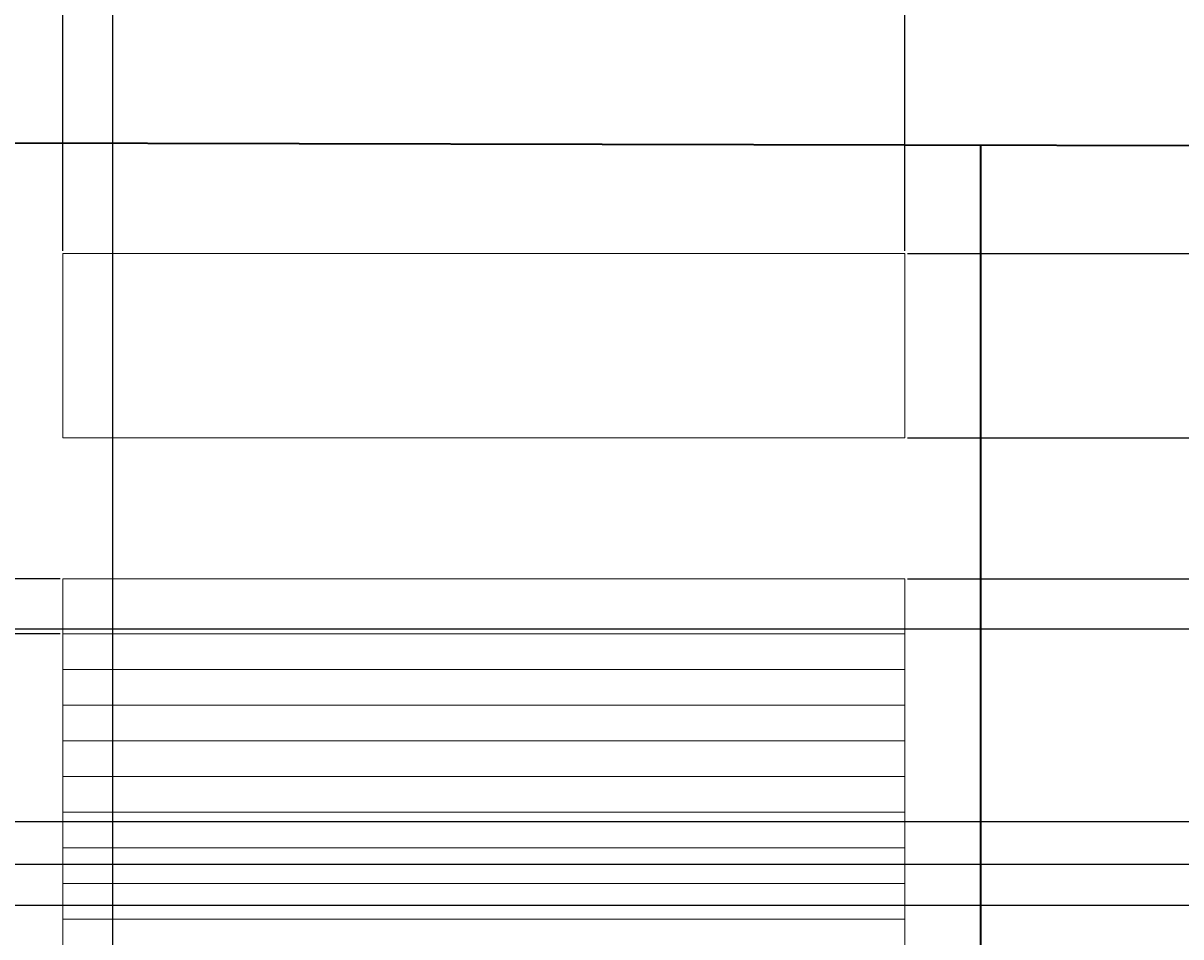
# Model space of a CAD drawing. Units: inches. Extents: x 27 to 200, y -50 to 102.
# Tile 13 of 26: x 144 to 172, y -3 to 19. Entities that reach past the tile are written whole.
import ezdxf

# ---------------------------------------------------------------- set-up
doc = ezdxf.new("R2010")
doc.units = ezdxf.units.IN
doc.header["$MEASUREMENT"] = 0
for name, color, linetype, lineweight in [('A-ANNO-DIMS', 2, 'Continuous', 18), ('A-ELEV', 7, 'Continuous', 35), ('A-EQPM', 9, 'Continuous', 18), ('A-FURN', 8, 'Continuous', 18)]:
    doc.layers.add(name, color=color, linetype=linetype, lineweight=lineweight)
doc.styles.get("Standard").update_dxf_attribs({"font": 'arial.ttf'})
doc.dimstyles.get("Standard").update_dxf_attribs({"dimtxt": 0.18, "dimasz": 0.18, "dimexe": 0.18, "dimexo": 0.0625, "dimgap": 0.09, "dimtad": 0, "dimtih": 1, "dimtoh": 1, "dimdec": 4, "dimzin": 0, "dimdsep": 46, "dimtxsty": 'Standard', "dimcen": 0.09, "dimadec": 0, "dimazin": 0, "dimtfac": 1, "dimtdec": 4, "dimtofl": 0, "dimtmove": 0, "dimatfit": 3, "dimfxl": 1, "dimtolj": 1, "dimtzin": 0, "dimarcsym": 0})

# ---------------------------------------------------------------- blocks, each defined once
blk = doc.blocks.new('*D48')
at = {"layer": 'A-ANNO-DIMS', "color": 0, "lineweight": -2, "transparency": 16777216}
for p, q in [((84.479, 44.926), (199.797, 44.926)), ((199.617, 44.746), (199.617, 14.26)), ((199.617, -16.589), (199.617, 13.897)), ((84.479, -16.769), (199.797, -16.769))]:
    blk.add_line(p, q, dxfattribs=at)
at = {"layer": 'A-ANNO-DIMS', "color": 0, "transparency": 16777216}
for points in [[(199.587, 44.746), (199.647, 44.746), (199.617, 44.926)], [(199.587, -16.589), (199.647, -16.589), (199.617, -16.769)]]:
    blk.add_solid(points, dxfattribs=at)
at = {"layer": 'Defpoints', "color": 0, "transparency": 16777216}
for p in [(84.417, 44.926), (199.617, 44.926), (84.417, -16.769)]:
    blk.add_point(p, dxfattribs=at)
at = {"layer": 'A-ANNO-DIMS', "color": 0, "transparency": 16777216, "insert": (199.617, 14.079), "char_height": 0.18, "attachment_point": 5}
blk.add_mtext('\\A1;61.7', dxfattribs=at)
blk = doc.blocks.new('*D51')
at = {"layer": 'A-ANNO-DIMS', "color": 0, "lineweight": -2, "transparency": 16777216}
for p, q in [((120.417, 45.561), (120.417, -25.149)), ((146.417, 45.561), (146.417, -25.149)), ((120.597, -24.969), (133.197, -24.969)), ((146.237, -24.969), (133.637, -24.969))]:
    blk.add_line(p, q, dxfattribs=at)
at = {"layer": 'A-ANNO-DIMS', "color": 0, "transparency": 16777216}
for points in [[(120.597, -24.939), (120.597, -24.999), (120.417, -24.969)], [(146.237, -24.939), (146.237, -24.999), (146.417, -24.969)]]:
    blk.add_solid(points, dxfattribs=at)
at = {"layer": 'Defpoints', "color": 0, "transparency": 16777216}
for p in [(120.417, 45.623), (146.417, 45.623), (146.417, -24.969)]:
    blk.add_point(p, dxfattribs=at)
at = {"layer": 'A-ANNO-DIMS', "color": 0, "transparency": 16777216, "insert": (133.417, -24.969), "char_height": 0.18, "attachment_point": 5}
blk.add_mtext('\\A1;26', dxfattribs=at)
blk = doc.blocks.new('*D58')
at = {"layer": 'A-ANNO-DIMS', "color": 0, "lineweight": -2, "transparency": 16777216}
for p, q in [((140.203, 4.418), (199.797, 4.418)), ((199.617, 4.238), (199.617, 1.273)), ((199.617, -2.056), (199.617, 0.909)), ((140.203, -2.236), (199.797, -2.236))]:
    blk.add_line(p, q, dxfattribs=at)
at = {"layer": 'A-ANNO-DIMS', "color": 0, "transparency": 16777216}
for points in [[(199.587, 4.238), (199.647, 4.238), (199.617, 4.418)], [(199.587, -2.056), (199.647, -2.056), (199.617, -2.236)]]:
    blk.add_solid(points, dxfattribs=at)
at = {"layer": 'Defpoints', "color": 0, "transparency": 16777216}
for p in [(140.141, 4.418), (199.617, 4.418), (140.141, -2.236)]:
    blk.add_point(p, dxfattribs=at)
at = {"layer": 'A-ANNO-DIMS', "color": 0, "transparency": 16777216, "insert": (199.617, 1.091), "char_height": 0.18, "attachment_point": 5}
blk.add_mtext('\\A1;6.654', dxfattribs=at)
blk = doc.blocks.new('*D60')
at = {"layer": 'A-ANNO-DIMS', "color": 0, "lineweight": -2, "transparency": 16777216}
for p, q in [((135.04, -0.225), (199.797, -0.225)), ((199.617, -0.405), (199.617, -0.559)), ((199.617, -1.076), (199.617, -0.923)), ((135.04, -1.256), (199.797, -1.256))]:
    blk.add_line(p, q, dxfattribs=at)
at = {"layer": 'A-ANNO-DIMS', "color": 0, "transparency": 16777216}
for points in [[(199.587, -0.405), (199.647, -0.405), (199.617, -0.225)], [(199.587, -1.076), (199.647, -1.076), (199.617, -1.256)]]:
    blk.add_solid(points, dxfattribs=at)
at = {"layer": 'Defpoints', "color": 0, "transparency": 16777216}
for p in [(134.978, -0.225), (199.617, -0.225), (134.978, -1.256)]:
    blk.add_point(p, dxfattribs=at)
at = {"layer": 'A-ANNO-DIMS', "color": 0, "transparency": 16777216, "insert": (199.617, -0.741), "char_height": 0.18, "attachment_point": 5}
blk.add_mtext('\\A1;1.03', dxfattribs=at)
blk = doc.blocks.new('*D64')
at = {"layer": 'A-ANNO-DIMS', "color": 0, "lineweight": -2, "transparency": 16777216}
for p, q in [((145.216, 13.517), (145.216, 102.306)), ((165.483, 13.517), (165.483, 102.306)), ((145.396, 102.126), (154.884, 102.126)), ((165.303, 102.126), (155.815, 102.126))]:
    blk.add_line(p, q, dxfattribs=at)
at = {"layer": 'A-ANNO-DIMS', "color": 0, "transparency": 16777216}
for points in [[(145.396, 102.156), (145.396, 102.096), (145.216, 102.126)], [(165.303, 102.156), (165.303, 102.096), (165.483, 102.126)]]:
    blk.add_solid(points, dxfattribs=at)
at = {"layer": 'Defpoints', "color": 0, "transparency": 16777216}
for p in [(165.483, 102.126), (145.216, 13.455), (165.483, 13.455)]:
    blk.add_point(p, dxfattribs=at)
at = {"layer": 'A-ANNO-DIMS', "color": 0, "transparency": 16777216, "insert": (155.35, 102.126), "char_height": 0.18, "attachment_point": 5}
blk.add_mtext('\\A1;20.267', dxfattribs=at)
blk = doc.blocks.new('*D65')
at = {"layer": 'A-ANNO-DIMS', "color": 0, "lineweight": -2, "transparency": 16777216}
for p, q in [((165.546, 13.455), (199.797, 13.455)), ((199.617, 13.275), (199.617, 11.414)), ((199.617, 9.193), (199.617, 11.054)), ((165.546, 9.013), (199.797, 9.013))]:
    blk.add_line(p, q, dxfattribs=at)
at = {"layer": 'A-ANNO-DIMS', "color": 0, "transparency": 16777216}
for points in [[(199.587, 13.275), (199.647, 13.275), (199.617, 13.455)], [(199.587, 9.193), (199.647, 9.193), (199.617, 9.013)]]:
    blk.add_solid(points, dxfattribs=at)
at = {"layer": 'Defpoints', "color": 0, "transparency": 16777216}
for p in [(165.483, 13.455), (199.617, 13.455), (165.483, 9.013)]:
    blk.add_point(p, dxfattribs=at)
at = {"layer": 'A-ANNO-DIMS', "color": 0, "transparency": 16777216, "insert": (199.617, 11.234), "char_height": 0.18, "attachment_point": 5}
blk.add_mtext('\\A1;4.442', dxfattribs=at)
blk = doc.blocks.new('*D67')
at = {"layer": 'A-ANNO-DIMS', "color": 0, "lineweight": -2, "transparency": 16777216}
for p, q in [((165.546, 5.617), (199.797, 5.617)), ((199.617, 5.437), (199.617, -3.019)), ((199.617, -11.839), (199.617, -3.383)), ((165.546, -12.019), (199.797, -12.019))]:
    blk.add_line(p, q, dxfattribs=at)
at = {"layer": 'A-ANNO-DIMS', "color": 0, "transparency": 16777216}
for points in [[(199.587, 5.437), (199.647, 5.437), (199.617, 5.617)], [(199.587, -11.839), (199.647, -11.839), (199.617, -12.019)]]:
    blk.add_solid(points, dxfattribs=at)
at = {"layer": 'Defpoints', "color": 0, "transparency": 16777216}
for p in [(165.484, 5.617), (199.617, 5.617), (165.484, -12.019)]:
    blk.add_point(p, dxfattribs=at)
at = {"layer": 'A-ANNO-DIMS', "color": 0, "transparency": 16777216, "insert": (199.617, -3.201), "char_height": 0.18, "attachment_point": 5}
blk.add_mtext('\\A1;17.636', dxfattribs=at)
blk = doc.blocks.new('*D68')
at = {"layer": 'A-ANNO-DIMS', "color": 0, "lineweight": -2, "transparency": 16777216}
for p, q in [((145.153, 5.617), (27.037, 5.617)), ((27.217, 5.437), (27.217, 5.138)), ((27.217, 4.476), (27.217, 4.774)), ((145.153, 4.296), (27.037, 4.296))]:
    blk.add_line(p, q, dxfattribs=at)
at = {"layer": 'A-ANNO-DIMS', "color": 0, "transparency": 16777216}
for points in [[(27.187, 5.437), (27.247, 5.437), (27.217, 5.617)], [(27.187, 4.476), (27.247, 4.476), (27.217, 4.296)]]:
    blk.add_solid(points, dxfattribs=at)
at = {"layer": 'Defpoints', "color": 0, "transparency": 16777216}
for p in [(27.217, 5.617), (145.216, 5.617), (145.216, 4.296)]:
    blk.add_point(p, dxfattribs=at)
at = {"layer": 'A-ANNO-DIMS', "color": 0, "transparency": 16777216, "insert": (27.217, 4.956), "char_height": 0.18, "attachment_point": 5}
blk.add_mtext('\\A1;1.32', dxfattribs=at)

msp = doc.modelspace()

# ---------------------------------------------------------------- linework, layer by layer
at = {"layer": 'A-ELEV'}
for p, q in [((191.4102, 16.002), (89.3051, 16.2307)), ((167.3118, -16.7693), (167.3118, 16.056))]:
    msp.add_line(p, q, dxfattribs=at)
at = {"layer": 'A-EQPM'}
for p, q in [((145.216, 4.2959), (165.4839, 4.2959)), ((145.216, 3.4373), (165.4839, 3.4373)), ((145.216, 2.5786), (165.4839, 2.5786)), ((145.216, 1.7199), (165.4839, 1.7199)), ((145.216, 0.8612), (165.4839, 0.8612)), ((145.216, 0.0025), (165.4839, 0.0025)), ((145.216, -0.8562), (165.4839, -0.8562)), ((145.216, -1.7148), (165.4839, -1.7148)), ((145.216, -2.5735), (165.4839, -2.5735))]:
    msp.add_line(p, q, dxfattribs=at)
at = {"layer": 'A-FURN'}
for points in [[(145.216, 13.4548), (165.4832, 13.4548), (165.4832, 9.0132), (145.216, 9.0132)], [(145.216, 5.6167), (165.4839, 5.6167), (165.4839, -12.0191), (145.216, -12.0191)]]:
    msp.add_lwpolyline(points, close=True, dxfattribs=at)

# ---------------------------------------------------------------- dimensions: what is measured, and where the dimension line sits
at = {"layer": 'A-ANNO-DIMS'}
for base, p1, p2, override, picture, middle in [((165.4832, 102.1264), (145.216, 13.4548), (165.4832, 13.4548), {"dimdec": 3, "dimlfac": 1, "dimrnd": 0, "dimzin": 0, "dimdsep": 46, "dimlunit": 2}, '*D64', (155.3496, 102.1264)), ((146.4169, -24.9693), (120.4169, 45.6231), (146.4169, 45.6231), {"dimdec": 0, "dimlfac": 1, "dimrnd": 0, "dimzin": 0, "dimdsep": 46, "dimlunit": 2}, '*D51', (133.4169, -24.9693))]:
    dim = msp.add_linear_dim(base=base, p1=p1, p2=p2, dimstyle='Standard', override=override, dxfattribs=at)
    dim.commit()
    dim.dimension.update_dxf_attribs({"geometry": picture, "text_midpoint": middle})
for base, p1, p2, override, picture, middle in [((199.6169, 44.9264), (84.4169, -16.7693), (84.4169, 44.9264), {"dimdec": 1, "dimlfac": 1, "dimrnd": 0, "dimzin": 0, "dimdsep": 46, "dimlunit": 2}, '*D48', (199.6169, 14.0786)), ((199.6169, 13.4548), (165.4832, 9.0132), (165.4832, 13.4548), {"dimdec": 3, "dimlfac": 1, "dimrnd": 0, "dimzin": 0, "dimdsep": 46, "dimlunit": 2}, '*D65', (199.6169, 11.234)), ((27.2169, 5.6167), (145.216, 4.2959), (145.216, 5.6167), {"dimdec": 2, "dimlfac": 1, "dimrnd": 0, "dimzin": 0, "dimdsep": 46, "dimlunit": 2}, '*D68', (27.2169, 4.9563)), ((199.6169, 5.6167), (165.4839, -12.0191), (165.4839, 5.6167), {"dimdec": 3, "dimlfac": 1, "dimrnd": 0, "dimzin": 0, "dimdsep": 46, "dimlunit": 2}, '*D67', (199.6169, -3.2012)), ((199.6169, 4.4177), (140.1406, -2.2364), (140.1406, 4.4177), {"dimdec": 3, "dimlfac": 1, "dimrnd": 0, "dimzin": 0, "dimdsep": 46, "dimlunit": 2}, '*D58', (199.6169, 1.0906)), ((199.6169, -0.2247), (134.9776, -1.2564), (134.9776, -0.2247), {"dimdec": 2, "dimlfac": 1, "dimrnd": 0, "dimzin": 0, "dimdsep": 46, "dimlunit": 2}, '*D60', (199.6169, -0.7405))]:
    dim = msp.add_linear_dim(base=base, p1=p1, p2=p2, angle=90, dimstyle='Standard', override=override, dxfattribs=at)
    dim.commit()
    dim.dimension.update_dxf_attribs({"geometry": picture, "text_midpoint": middle})

doc.saveas('drawing.dxf')
